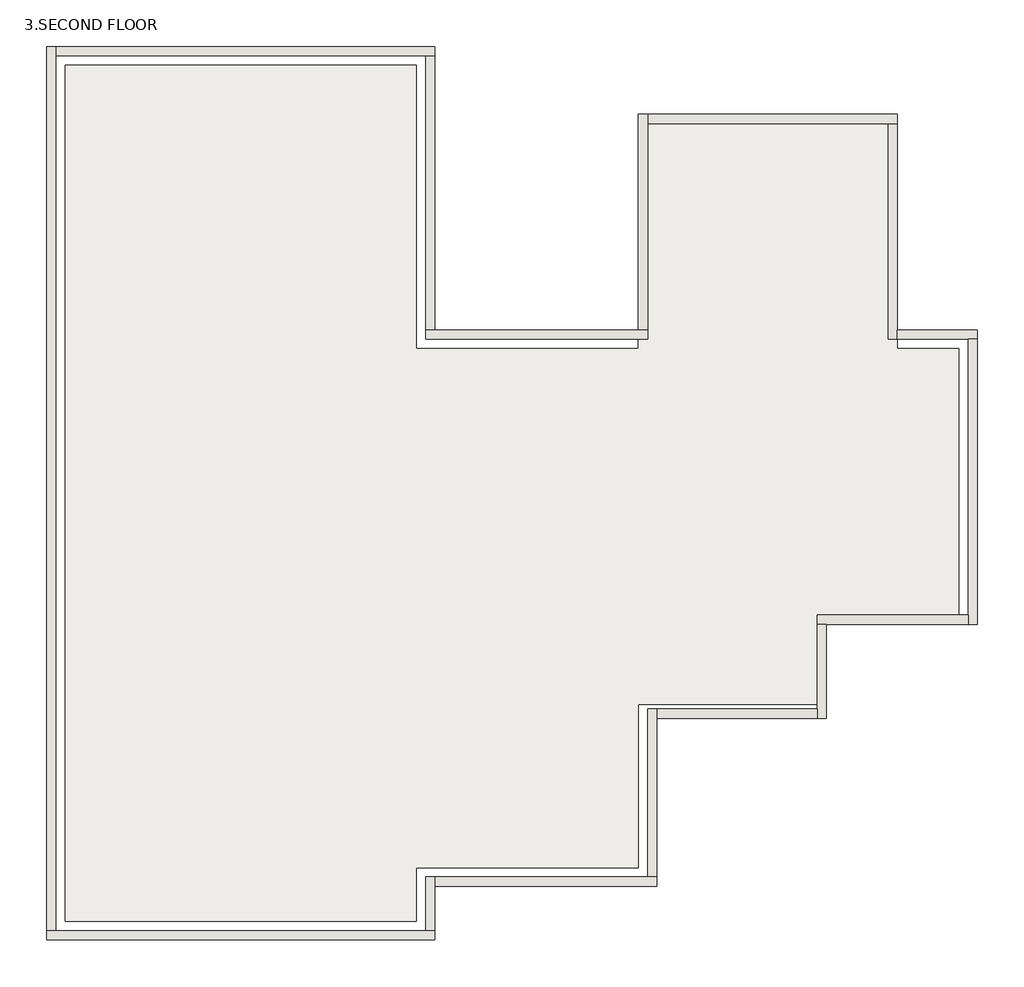
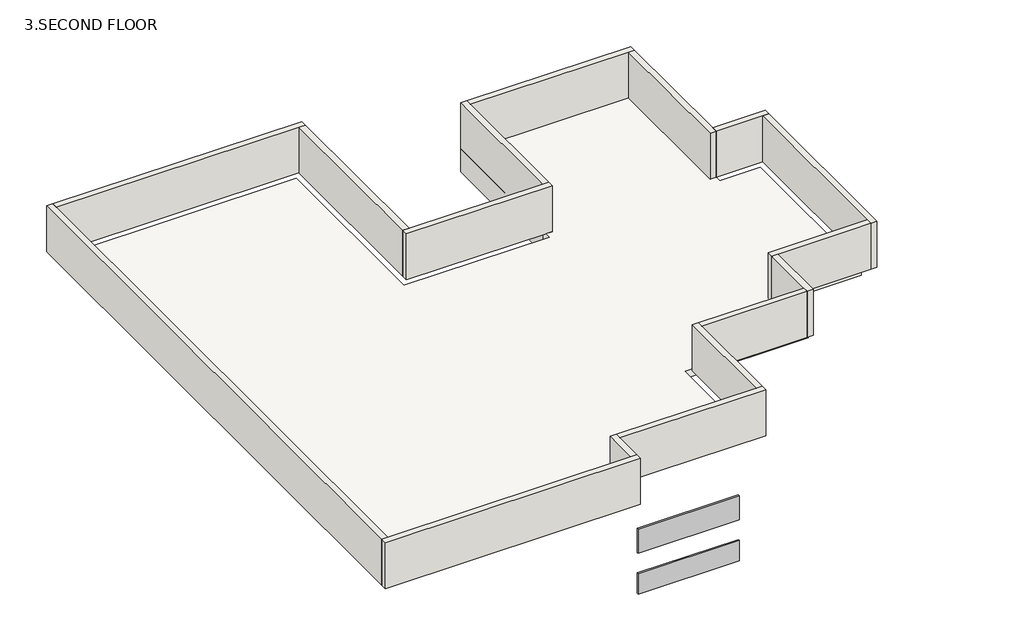
# One storey: 16 walls, 2 plates, 1 slab.
"""IFC4 building model written with IfcOpenShell, lengths in millimetres."""

from ifc_helpers import new_model, si_unit, frame, origin, place, context, project, spatial, polyline, outline, extrude, faceted_brep, transform, mapped, element, save
from components import system_panel_glazed_df97d9fa, system_panel_glazed_db63c8d7

model = new_model("IFC4")

# Units and contexts
model_context = context("Model", 3, world=origin())
ifc_project = project(units=[si_unit("LENGTHUNIT", "METRE", prefix="MILLI")], contexts=[model_context])

# Site, building, storey
site = spatial("IfcSite", under=ifc_project)
building = spatial("IfcBuilding", under=site)
storey = spatial("IfcBuildingStorey", under=building, Name="3.SECOND FLOOR", Elevation=7010.4)

# Plates
placement = place(None, origin())
system_panel_glazed_shape = system_panel_glazed_df97d9fa(model_context)
element("IfcPlate", 1, ObjectType="System Panel : Glazed", at=placement, inside=storey, context=model_context, shape_type="MappedRepresentation", body=[
    mapped(system_panel_glazed_shape, transform((-1429.2657257, 2.5160289, 5446.3786483), x_axis=(1.0, 0.0, 0.0), y_axis=(0.0, 1.0, 0.0), z_axis=(0.0, 0.0, 1.0))),
])
system_panel_glazed_2_shape = system_panel_glazed_db63c8d7(model_context)
element("IfcPlate", 2, ObjectType="System Panel : Glazed", at=placement, inside=storey, context=model_context, shape_type="MappedRepresentation", body=[
    mapped(system_panel_glazed_2_shape, transform((-1429.2657257, 2.5160289, 4633.507951), x_axis=(1.0, 0.0, 0.0), y_axis=(0.0, 1.0, 0.0), z_axis=(0.0, 0.0, 1.0))),
])

# Slab
element("IfcSlab", 3, ObjectType="6\" FLOOR", at=placement, inside=storey, context=model_context, shape_type="SweptSolid", body=[
    extrude(outline(polyline([(-2993.0749552, 10099.0160289), (-2993.0749552, 6593.8160289), (-249.8749552, 6593.8160289), (-249.8749552, 9489.4160289), (2950.5250448, 9489.4160289), (2950.5250448, 6708.1160289), (2950.5250448, 6593.8160289), (3712.5250448, 6593.8160289), (3712.5250448, 3298.1660289), (2074.2250448, 3298.1660289), (2074.2250448, 2193.2660289), (-249.8749552, 2193.2660289), (-249.8749552, 173.9660289), (-2993.0749552, 173.9660289), (-2993.0749552, -492.7839711), (-7336.4749552, -492.7839711), (-7336.4749552, 10099.0160289), (-2993.0749552, 10099.0160289)])), frame((0.0, 0.0, 6858.0), z_axis=(0.0, 0.0, 1.0), x_axis=(1.0, 0.0, 0.0)), (0.0, 0.0, 1.0), 152.4),
])

# Walls
element("IfcWall", 4, ObjectType="4.5\" wall", at=placement, inside=storey, context=model_context, shape_type="Brep", body=[
    faceted_brep([(-7565.0749552, -721.3839711, 7010.4), (-2764.4749552, -721.3839711, 7010.4), (-2764.4749552, -721.3839711, 7924.8), (-7565.0749552, -721.3839711, 7924.8), (-7565.0749552, -607.0839711, 7010.4), (-7565.0749552, -607.0839711, 7924.8), (-7450.7749552, -607.0839711, 7924.8), (-2878.7749552, -607.0839711, 7924.8), (-2764.4749552, -607.0839711, 7924.8), (-2764.4749552, -607.0839711, 7010.4), (-2878.7749552, -607.0839711, 7010.4), (-7450.7749552, -607.0839711, 7010.4)], [[[0, 1, 2, 3]], [[4, 5, 6, 7, 8, 9, 10, 11]], [[1, 0, 4, 11, 10, 9]], [[3, 2, 8, 7, 6, 5]], [[2, 1, 9, 8]], [[0, 3, 5, 4]]]),
])
element("IfcWall", 5, ObjectType="4.5\" wall", at=placement, inside=storey, context=model_context, shape_type="Brep", body=[
    faceted_brep([(-7450.7749552, -607.0839711, 7010.4), (-7450.7749552, 10213.3160289, 7010.4), (-7450.7749552, 10327.6160289, 7010.4), (-7450.7749552, 10327.6160289, 7924.8), (-7450.7749552, 10213.3160289, 7924.8), (-7450.7749552, -607.0839711, 7924.8), (-7565.0749552, -607.0839711, 7010.4), (-7565.0749552, -607.0839711, 7924.8), (-7565.0749552, 10327.6160289, 7924.8), (-7565.0749552, 10327.6160289, 7010.4)], [[[0, 1, 2, 3, 4, 5]], [[6, 7, 8, 9]], [[2, 1, 0, 6, 9]], [[5, 4, 3, 8, 7]], [[0, 5, 7, 6]], [[3, 2, 9, 8]]]),
])
element("IfcWall", 6, ObjectType="4.5\" wall", at=placement, inside=storey, context=model_context, shape_type="Brep", body=[
    faceted_brep([(-7450.7749552, 10213.3160289, 7010.4), (-2878.7749552, 10213.3160289, 7010.4), (-2764.4749552, 10213.3160289, 7010.4), (-2764.4749552, 10213.3160289, 7924.8), (-2878.7749552, 10213.3160289, 7924.8), (-7450.7749552, 10213.3160289, 7924.8), (-7450.7749552, 10327.6160289, 7010.4), (-7450.7749552, 10327.6160289, 7924.8), (-2764.4749552, 10327.6160289, 7924.8), (-2764.4749552, 10327.6160289, 7010.4)], [[[0, 1, 2, 3, 4, 5]], [[6, 7, 8, 9]], [[2, 1, 0, 6, 9]], [[5, 4, 3, 8, 7]], [[3, 2, 9, 8]], [[0, 5, 7, 6]]]),
])
element("IfcWall", 7, ObjectType="4.5\" wall", at=placement, inside=storey, context=model_context, shape_type="Brep", body=[
    faceted_brep([(-2878.7749552, 6708.1160289, 7010.4), (-192.7249552, 6708.1160289, 7010.4), (-135.5749552, 6708.1160289, 7010.4), (-135.5749552, 6708.1160289, 7924.8), (-2878.7749552, 6708.1160289, 7924.8), (-2878.7749552, 6822.4160289, 7010.4), (-2878.7749552, 6822.4160289, 7924.8), (-2764.4749552, 6822.4160289, 7924.8), (-249.8749552, 6822.4160289, 7924.8), (-135.5749552, 6822.4160289, 7924.8), (-135.5749552, 6822.4160289, 7010.4), (-192.7249552, 6822.4160289, 7010.4), (-2764.4749552, 6822.4160289, 7010.4)], [[[0, 1, 2, 3, 4]], [[5, 6, 7, 8, 9, 10, 11, 12]], [[2, 1, 0, 5, 12, 11, 10]], [[4, 3, 9, 8, 7, 6]], [[0, 4, 6, 5]], [[3, 2, 10, 9]]]),
])
element("IfcWall", 8, ObjectType="4.5\" wall", at=placement, inside=storey, context=model_context, shape_type="SweptSolid", body=[
    extrude(outline(polyline([(-2764.4749552, 10213.3160289), (-2764.4749552, 6822.4160289), (-2878.7749552, 6822.4160289), (-2878.7749552, 10213.3160289), (-2764.4749552, 10213.3160289)])), frame((0.0, 0.0, 7010.4), z_axis=(0.0, 0.0, 1.0), x_axis=(1.0, 0.0, 0.0)), (0.0, 0.0, 1.0), 914.4),
])
element("IfcWall", 9, ObjectType="4.5\" wall", at=placement, inside=storey, context=model_context, shape_type="Brep", body=[
    faceted_brep([(-135.5749552, 6708.1160289, 6553.2), (-135.5749552, 9375.1160289, 6553.2), (-135.5749552, 9489.4160289, 6553.2), (-135.5749552, 9489.4160289, 7924.8), (-135.5749552, 9375.1160289, 7924.8), (-135.5749552, 6822.4160289, 7924.8), (-135.5749552, 6822.4160289, 7010.4), (-135.5749552, 6708.1160289, 7010.4), (-249.8749552, 6822.4160289, 6553.2), (-249.8749552, 6822.4160289, 7010.4), (-249.8749552, 6822.4160289, 7924.8), (-249.8749552, 9489.4160289, 7924.8), (-249.8749552, 9489.4160289, 6553.2), (-192.7249552, 6708.1160289, 6553.2), (-192.7249552, 6822.4160289, 6553.2), (-192.7249552, 6822.4160289, 7010.4), (-192.7249552, 6708.1160289, 7010.4)], [[[0, 1, 2, 3, 4, 5, 6, 7]], [[8, 9, 10, 11, 12]], [[2, 1, 0, 13, 14, 8, 12]], [[5, 4, 3, 11, 10]], [[3, 2, 12, 11]], [[6, 15, 16, 7]], [[0, 7, 16, 13]], [[16, 15, 14, 13]], [[15, 9, 8, 14]], [[6, 5, 10, 9, 15]]]),
])
element("IfcWall", 10, ObjectType="4.5\" wall", at=placement, inside=storey, context=model_context, shape_type="Brep", body=[
    faceted_brep([(-135.5749552, 9375.1160289, 6553.2), (2836.2250448, 9375.1160289, 6553.2), (2950.5250448, 9375.1160289, 6553.2), (2950.5250448, 9375.1160289, 7924.8), (2836.2250448, 9375.1160289, 7924.8), (-135.5749552, 9375.1160289, 7924.8), (-135.5749552, 9489.4160289, 6553.2), (-135.5749552, 9489.4160289, 7924.8), (2950.5250448, 9489.4160289, 7924.8), (2950.5250448, 9489.4160289, 6553.2)], [[[0, 1, 2, 3, 4, 5]], [[6, 7, 8, 9]], [[2, 1, 0, 6, 9]], [[5, 4, 3, 8, 7]], [[3, 2, 9, 8]], [[0, 5, 7, 6]]]),
])
element("IfcWall", 11, ObjectType="4.5\" wall", at=placement, inside=storey, context=model_context, shape_type="Brep", body=[
    faceted_brep([(2836.2250448, 9375.1160289, 6553.2), (2836.2250448, 6708.1160289, 6553.2), (2836.2250448, 6708.1160289, 7924.8), (2836.2250448, 9375.1160289, 7924.8), (2950.5250448, 9375.1160289, 6553.2), (2950.5250448, 9375.1160289, 7924.8), (2950.5250448, 6822.4160289, 7924.8), (2950.5250448, 6708.1160289, 7924.8), (2950.5250448, 6708.1160289, 7010.4), (2950.5250448, 6708.1160289, 6553.2)], [[[0, 1, 2, 3]], [[4, 5, 6, 7, 8, 9]], [[1, 0, 4, 9]], [[3, 2, 7, 6, 5]], [[0, 3, 5, 4]], [[2, 1, 9, 8, 7]]]),
])
element("IfcWall", 12, ObjectType="4.5\" wall", at=placement, inside=storey, context=model_context, shape_type="Brep", body=[
    faceted_brep([(3941.1250448, 6822.4160289, 7010.4), (2950.5250448, 6822.4160289, 7010.4), (2950.5250448, 6822.4160289, 7924.8), (3941.1250448, 6822.4160289, 7924.8), (3941.1250448, 6708.1160289, 7010.4), (3941.1250448, 6708.1160289, 7924.8), (3826.8250448, 6708.1160289, 7924.8), (2950.5250448, 6708.1160289, 7924.8), (2950.5250448, 6708.1160289, 7010.4), (3826.8250448, 6708.1160289, 7010.4)], [[[0, 1, 2, 3]], [[4, 5, 6, 7, 8, 9]], [[1, 0, 4, 9, 8]], [[3, 2, 7, 6, 5]], [[0, 3, 5, 4]], [[2, 1, 8, 7]]]),
])
element("IfcWall", 13, ObjectType="4.5\" wall", at=placement, inside=storey, context=model_context, shape_type="Brep", body=[
    faceted_brep([(3826.8250448, 6708.1160289, 7010.4), (3826.8250448, 3298.1660289, 7010.4), (3826.8250448, 3183.8660289, 7010.4), (3826.8250448, 3183.8660289, 7924.8), (3826.8250448, 3298.1660289, 7924.8), (3826.8250448, 6708.1160289, 7924.8), (3941.1250448, 6708.1160289, 7010.4), (3941.1250448, 6708.1160289, 7924.8), (3941.1250448, 3183.8660289, 7924.8), (3941.1250448, 3183.8660289, 7010.4)], [[[0, 1, 2, 3, 4, 5]], [[6, 7, 8, 9]], [[2, 1, 0, 6, 9]], [[5, 4, 3, 8, 7]], [[3, 2, 9, 8]], [[0, 5, 7, 6]]]),
])
element("IfcWall", 14, ObjectType="4.5\" wall", at=placement, inside=storey, context=model_context, shape_type="Brep", body=[
    faceted_brep([(3826.8250448, 3298.1660289, 7010.4), (1959.9250448, 3298.1660289, 7010.4), (1959.9250448, 3298.1660289, 7924.8), (3826.8250448, 3298.1660289, 7924.8), (3826.8250448, 3183.8660289, 7010.4), (3826.8250448, 3183.8660289, 7924.8), (2074.2250448, 3183.8660289, 7924.8), (1959.9250448, 3183.8660289, 7924.8), (1959.9250448, 3183.8660289, 7010.4), (2074.2250448, 3183.8660289, 7010.4)], [[[0, 1, 2, 3]], [[4, 5, 6, 7, 8, 9]], [[1, 0, 4, 9, 8]], [[3, 2, 7, 6, 5]], [[2, 1, 8, 7]], [[0, 3, 5, 4]]]),
])
element("IfcWall", 15, ObjectType="4.5\" wall", at=placement, inside=storey, context=model_context, shape_type="Brep", body=[
    faceted_brep([(1959.9250448, 3183.8660289, 7010.4), (1959.9250448, 2136.1160289, 7010.4), (1959.9250448, 2021.8160289, 7010.4), (1959.9250448, 2021.8160289, 7924.8), (1959.9250448, 2136.1160289, 7924.8), (1959.9250448, 3183.8660289, 7924.8), (2074.2250448, 3183.8660289, 7010.4), (2074.2250448, 3183.8660289, 7924.8), (2074.2250448, 2021.8160289, 7924.8), (2074.2250448, 2021.8160289, 7010.4)], [[[0, 1, 2, 3, 4, 5]], [[6, 7, 8, 9]], [[2, 1, 0, 6, 9]], [[5, 4, 3, 8, 7]], [[3, 2, 9, 8]], [[0, 5, 7, 6]]]),
])
element("IfcWall", 16, ObjectType="4.5\" wall", at=placement, inside=storey, context=model_context, shape_type="Brep", body=[
    faceted_brep([(-2764.4749552, -607.0839711, 7010.4), (-2764.4749552, -54.6339711, 7010.4), (-2764.4749552, 59.6660289, 7010.4), (-2764.4749552, 59.6660289, 7924.8), (-2764.4749552, -54.6339711, 7924.8), (-2764.4749552, -607.0839711, 7924.8), (-2878.7749552, -607.0839711, 7010.4), (-2878.7749552, -607.0839711, 7924.8), (-2878.7749552, 59.6660289, 7924.8), (-2878.7749552, 59.6660289, 7010.4)], [[[0, 1, 2, 3, 4, 5]], [[6, 7, 8, 9]], [[2, 1, 0, 6, 9]], [[5, 4, 3, 8, 7]], [[3, 2, 9, 8]], [[0, 5, 7, 6]]]),
])
element("IfcWall", 17, ObjectType="4.5\" wall", at=placement, inside=storey, context=model_context, shape_type="Brep", body=[
    faceted_brep([(-2764.4749552, -54.6339711, 7010.4), (-21.2749552, -54.6339711, 7010.4), (-21.2749552, -54.6339711, 7924.8), (-2764.4749552, -54.6339711, 7924.8), (-2764.4749552, 59.6660289, 7010.4), (-2764.4749552, 59.6660289, 7924.8), (-135.5749552, 59.6660289, 7924.8), (-21.2749552, 59.6660289, 7924.8), (-21.2749552, 59.6660289, 7010.4), (-135.5749552, 59.6660289, 7010.4)], [[[0, 1, 2, 3]], [[4, 5, 6, 7, 8, 9]], [[1, 0, 4, 9, 8]], [[3, 2, 7, 6, 5]], [[0, 3, 5, 4]], [[2, 1, 8, 7]]]),
])
element("IfcWall", 18, ObjectType="4.5\" wall", at=placement, inside=storey, context=model_context, shape_type="Brep", body=[
    faceted_brep([(-21.2749552, 59.6660289, 7010.4), (-21.2749552, 2021.8160289, 7010.4), (-21.2749552, 2136.1160289, 7010.4), (-21.2749552, 2136.1160289, 7924.8), (-21.2749552, 2021.8160289, 7924.8), (-21.2749552, 59.6660289, 7924.8), (-135.5749552, 59.6660289, 7010.4), (-135.5749552, 59.6660289, 7924.8), (-135.5749552, 2136.1160289, 7924.8), (-135.5749552, 2136.1160289, 7010.4)], [[[0, 1, 2, 3, 4, 5]], [[6, 7, 8, 9]], [[2, 1, 0, 6, 9]], [[5, 4, 3, 8, 7]], [[0, 5, 7, 6]], [[3, 2, 9, 8]]]),
])
element("IfcWall", 19, ObjectType="4.5\" wall", at=placement, inside=storey, context=model_context, shape_type="SweptSolid", body=[
    extrude(outline(polyline([(-21.2749552, 2136.1160289), (1959.9250448, 2136.1160289), (1959.9250448, 2021.8160289), (-21.2749552, 2021.8160289), (-21.2749552, 2136.1160289)])), frame((0.0, 0.0, 7010.4), z_axis=(0.0, 0.0, 1.0), x_axis=(1.0, 0.0, 0.0)), (0.0, 0.0, 1.0), 914.4),
])

save(model, "model.ifc")

# Revit data of these elements
# Type "System Panel : Glazed"
#   Construction Type Id = "GSP4R"
#   Analytic Construction = "1/8 in Pilkington single glazing"
#   Visual Light Transmittance = 0.9
#   Solar Heat Gain Coefficient = 0.86
#   Heat Transfer Coefficient (U) = 1.18115 BTU/(h·ft²·°F)
#   Define Thermal Properties by = 1
# Type "6\" FLOOR"
#   Assembly Code = "B1010"
#   Function = 0
#   Layers, outside or top first: 0' - 6" "Gypsum Wall Board" (function 1)
# Type "4.5\" wall"
#   Assembly Code = "B2010"
#   Layers, outside or top first: 0' - 4 1/2" "Gypsum Wall Board" (function 1)
# Elements 1, 2 (IfcPlate, "System Panel : Glazed")
#   Phase Created = New Construction
#   Materials on its faces: "Glass"
# Element 3 (IfcSlab, "6\" FLOOR")
#   Height Offset From Level = 0' - 0"
#   Phase Created = New Construction
#   Materials on its faces: "Gypsum Wall Board"
# Elements 4, 5, 6, 7, 8, 12, 13, 14, 15, 16, 17, 18, 19 (IfcWall, "4.5\" wall")
#   Top Offset = 0' - 0"
#   Base Offset = 0' - 0"
#   wall height = 3' - 0"
#   Phase Created = New Construction
#   Base Constraint = 3.SECOND FLOOR
#   Top Constraint = 4.PARAPET WALL
#   Materials on its faces: "Gypsum Wall Board"
# Elements 9, 10, 11 (IfcWall, "4.5\" wall")
#   built-in parameter 1001111 = -1' - 6"
#   Top Offset = 0' - 0"
#   Base Offset = -1' - 6"
#   wall height = 4' - 6"
#   Phase Created = New Construction
#   Base Constraint = 3.SECOND FLOOR
#   Top Constraint = 4.PARAPET WALL
#   Materials on its faces: "Gypsum Wall Board"
# Materials
#   "Gypsum Wall Board": class "Generic", colour RGB 228 228 228, transparency 0, Description = "Gypsum Wall Board", Cost = 0
#   "Glass": class "Glass", colour RGB 0 128 192, transparency 0.75, Description = "Soda Lime Glass", Cost = 0
